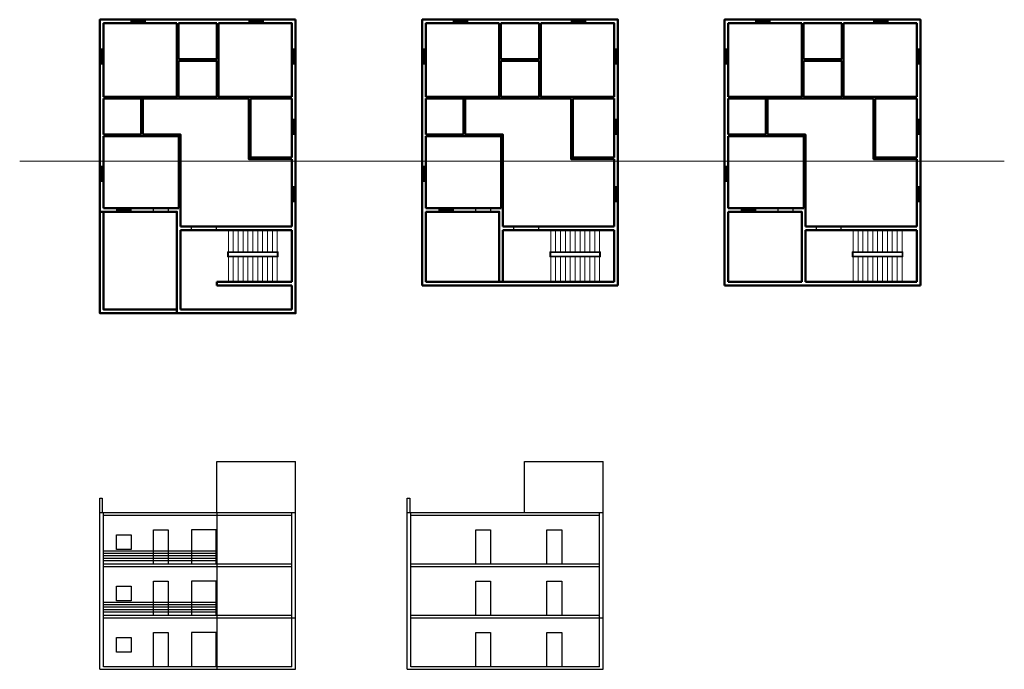
# Model space of a CAD drawing. Units: feet. Extents: x -965 to 1449, y -3391 to -1798.
import ezdxf

# ---------------------------------------------------------------- set-up
doc = ezdxf.new("R2010")
doc.units = ezdxf.units.FT
for name, color, linetype, lineweight in [('A-DOOR', 3, 'Continuous', 25), ('A-ELEV', 7, 'Continuous', 25), ('A-FLOR-STRS', 6, 'Continuous', 18), ('A-GLAZ', 4, 'Continuous', 25), ('A-GRID', 8, 'Continuous', 13), ('A-WALL', 7, 'Continuous', 50)]:
    doc.layers.add(name, color=color, linetype=linetype, lineweight=lineweight)

# ---------------------------------------------------------------- blocks, each defined once
blk = doc.blocks.new('WIN-1200')
for p, q in [((-765.9, -1906), (-765.9, -1870)), ((-764.2, -1906), (-764.2, -1870)), ((-762.5, -1906), (-762.5, -1870))]:
    blk.add_line(p, q)
blk.add_lwpolyline([(-768.7, -1906), (-759.7, -1906), (-759.7, -1870), (-768.7, -1870)], close=True)
blk = doc.blocks.new('ELEV-DOOR')
for p, q in [((0, 0), (0, 84)), ((0, 84), (36, 84)), ((36, 84), (36, 0))]:
    blk.add_line(p, q)
blk = doc.blocks.new('ELEV-WIN-SQ')
for p, q in [((0, 0), (0, 36)), ((0, 36), (36, 36)), ((36, 36), (36, 0)), ((36, 0), (0, 0))]:
    blk.add_line(p, q)
blk = doc.blocks.new('ELEV-DOOR-WIDE')
for p, q in [((60, 84), (0, 84)), ((0, 84), (0, 0)), ((60, 0), (60, 84))]:
    blk.add_line(p, q)

msp = doc.modelspace()

# ---------------------------------------------------------------- linework, layer by layer
at = {"layer": 'A-DOOR'}
for points in [[(-477.7, -1836.7), (-481.7, -1836.7), (-481.7, -1812.7), (-477.7, -1812.7)], [(312.6, -1836.7), (308.6, -1836.7), (308.6, -1812.7), (312.6, -1812.7)], [(1054.2, -1836.7), (1050.2, -1836.7), (1050.2, -1812.7), (1054.2, -1812.7)], [(-575.7, -1980.6), (-579.7, -1980.6), (-579.7, -1956.6), (-575.7, -1956.6)], [(214.6, -1980.6), (210.6, -1980.6), (210.6, -1956.6), (214.6, -1956.6)], [(956.2, -1980.6), (952.2, -1980.6), (952.2, -1956.6), (956.2, -1956.6)], [(-605, -1986.7), (-605, -1990.7), (-641, -1990.7), (-641, -1986.7)], [(-426.7, -1986.7), (-426.7, -1990.7), (-462.7, -1990.7), (-462.7, -1986.7)], [(185.3, -1986.7), (185.3, -1990.7), (149.3, -1990.7), (149.3, -1986.7)], [(363.6, -1986.7), (363.6, -1990.7), (327.6, -1990.7), (327.6, -1986.7)], [(926.9, -1986.7), (926.9, -1990.7), (890.9, -1990.7), (890.9, -1986.7)], [(1105.2, -1986.7), (1105.2, -1990.7), (1069.2, -1990.7), (1069.2, -1986.7)], [(-663.7, -2047.5), (-667.7, -2047.5), (-667.7, -2023.5), (-663.7, -2023.5)], [(126.6, -2047.5), (122.6, -2047.5), (122.6, -2023.5), (126.6, -2023.5)], [(868.2, -2047.5), (864.2, -2047.5), (864.2, -2023.5), (868.2, -2023.5)], [(-601.2, -2079.7), (-601.2, -2083.7), (-637.2, -2083.7), (-637.2, -2079.7)], [(-403.6, -2087.8), (-399.6, -2087.8), (-399.6, -2123.8), (-403.6, -2123.8)], [(189.1, -2079.7), (189.1, -2083.7), (153, -2083.7), (153, -2079.7)], [(386.7, -2087.8), (390.7, -2087.8), (390.7, -2123.8), (386.7, -2123.8)], [(930.6, -2079.7), (930.6, -2083.7), (894.6, -2083.7), (894.6, -2079.7)], [(1128.3, -2087.8), (1132.3, -2087.8), (1132.3, -2123.8), (1128.3, -2123.8)], [(-483.8, -2305.4), (-483.8, -2314.4), (-543.8, -2314.4), (-543.8, -2305.4)], [(306.5, -2305.4), (306.5, -2314.4), (246.5, -2314.4), (246.5, -2305.4)], [(1048.1, -2305.4), (1048.1, -2314.4), (988.1, -2314.4), (988.1, -2305.4)]]:
    msp.add_lwpolyline(points, close=True, dxfattribs=at)
for points in [[(-637.2, -2268.7), (-637.2, -2259.7), (-601.2, -2259.7), (-601.2, -2268.7)], [(153, -2268.7), (153, -2259.7), (189.1, -2259.7), (189.1, -2268.7)], [(894.6, -2268.7), (894.6, -2259.7), (930.6, -2259.7), (930.6, -2268.7)]]:
    msp.add_lwpolyline(points, dxfattribs=at)
at = {"layer": 'A-ELEV'}
for p, q in [((-481.5, -3007.2), (-481.5, -2881.2)), ((-481.5, -2881.2), (-288.7, -2881.2)), ((-288.7, -3391.2), (-288.7, -2881.2)), ((272.1, -3007.2), (272.1, -2881.2)), ((272.1, -2881.2), (465, -2881.2)), ((465, -3391.2), (465, -2881.2)), ((-768.7, -3007.2), (-768.7, -2971.2)), ((-768.7, -2971.2), (-762.7, -2971.2)), ((-762.7, -2971.2), (-762.7, -3007.2)), ((-15, -3007.2), (-15, -2971.2)), ((-15, -2971.2), (-9, -2971.2)), ((-9, -2971.2), (-9, -3007.2)), ((-288.7, -3007.2), (-768.7, -3007.2)), ((-768.7, -3391.2), (-768.7, -3007.2)), ((-759.7, -3385.2), (-759.7, -3007.2)), ((-759.7, -3013.2), (-297.7, -3013.2)), ((-481.5, -3007.2), (-481.5, -3391.2)), ((-297.7, -3385.2), (-297.7, -3007.2)), ((465, -3007.2), (-15, -3007.2)), ((-15, -3391.2), (-15, -3007.2)), ((-6, -3385.2), (-6, -3007.2)), ((-6, -3013.2), (456, -3013.2)), ((456, -3385.2), (456, -3007.2)), ((-481.5, -3124.9), (-759.7, -3124.9)), ((-297.7, -3133.2), (-759.7, -3133.2)), ((-297.7, -3133.2), (-759.7, -3133.2)), ((456, -3133.2), (-6, -3133.2)), ((456, -3133.2), (-6, -3133.2)), ((-759.7, -3139.2), (-297.7, -3139.2)), ((-759.7, -3139.2), (-297.7, -3139.2)), ((-6, -3139.2), (456, -3139.2)), ((-6, -3139.2), (456, -3139.2)), ((-481.5, -3250.9), (-759.7, -3250.9)), ((-297.7, -3259.2), (-759.7, -3259.2)), ((-297.7, -3259.2), (-759.7, -3259.2)), ((-759.7, -3265.2), (-288.7, -3265.2)), ((-759.7, -3265.2), (-297.7, -3265.2)), ((456, -3259.2), (-6, -3259.2)), ((456, -3259.2), (-6, -3259.2)), ((-6, -3265.2), (465, -3265.2)), ((-6, -3265.2), (456, -3265.2)), ((-768.7, -3391.2), (-288.7, -3391.2)), ((-297.7, -3385.2), (-759.7, -3385.2)), ((-15, -3391.2), (465, -3391.2)), ((456, -3385.2), (-6, -3385.2))]:
    msp.add_line(p, q, dxfattribs=at)
for points in [[(-481.5, -3107.3), (-759.7, -3107.3), (-759.7, -3100.3), (-481.5, -3100.3)], [(-481.5, -3119.1), (-759.7, -3119.1), (-759.7, -3112.2), (-481.5, -3112.2)], [(-481.5, -3233.3), (-759.7, -3233.3), (-759.7, -3226.3), (-481.5, -3226.3)], [(-481.5, -3245.1), (-759.7, -3245.1), (-759.7, -3238.2), (-481.5, -3238.2)]]:
    msp.add_lwpolyline(points, close=True, dxfattribs=at)
at = {"layer": 'A-FLOR-STRS'}
for p, q in [((-453.7, -2314.4), (-453.7, -2367.2)), ((-441.7, -2314.4), (-441.7, -2367.2)), ((-429.7, -2314.4), (-429.7, -2367.2)), ((-417.7, -2314.4), (-417.7, -2367.2)), ((-405.7, -2314.4), (-405.7, -2367.2)), ((-393.7, -2314.4), (-393.7, -2367.2)), ((-381.7, -2314.4), (-381.7, -2367.2)), ((-369.7, -2314.4), (-369.7, -2367.2)), ((-357.7, -2314.4), (-357.7, -2367.2)), ((-345.7, -2314.4), (-345.7, -2367.2)), ((-333.7, -2314.4), (-333.7, -2367.2)), ((336.6, -2314.4), (336.6, -2367.2)), ((348.6, -2314.4), (348.6, -2367.2)), ((360.6, -2314.4), (360.6, -2367.2)), ((372.6, -2314.4), (372.6, -2367.2)), ((384.6, -2314.4), (384.6, -2367.2)), ((396.6, -2314.4), (396.6, -2367.2)), ((408.6, -2314.4), (408.6, -2367.2)), ((420.6, -2314.4), (420.6, -2367.2)), ((432.6, -2314.4), (432.6, -2367.2)), ((444.6, -2314.4), (444.6, -2367.2)), ((456.6, -2314.4), (456.6, -2367.2)), ((1078.2, -2314.4), (1078.2, -2367.2)), ((1090.2, -2314.4), (1090.2, -2367.2)), ((1102.2, -2314.4), (1102.2, -2367.2)), ((1114.2, -2314.4), (1114.2, -2367.2)), ((1126.2, -2314.4), (1126.2, -2367.2)), ((1138.2, -2314.4), (1138.2, -2367.2)), ((1150.2, -2314.4), (1150.2, -2367.2)), ((1162.2, -2314.4), (1162.2, -2367.2)), ((1174.2, -2314.4), (1174.2, -2367.2)), ((1186.2, -2314.4), (1186.2, -2367.2)), ((1198.2, -2314.4), (1198.2, -2367.2)), ((-453.7, -2369.2), (-453.7, -2377.7)), ((-453.7, -2379.7), (-453.7, -2440.9)), ((-441.7, -2379.7), (-441.7, -2440.9)), ((-429.7, -2379.7), (-429.7, -2440.9)), ((-417.7, -2379.7), (-417.7, -2440.9)), ((-405.7, -2379.7), (-405.7, -2440.9)), ((-393.7, -2379.7), (-393.7, -2440.9)), ((-381.7, -2379.7), (-381.7, -2440.9)), ((-369.7, -2379.7), (-369.7, -2440.9)), ((-357.7, -2379.7), (-357.7, -2440.9)), ((-345.7, -2379.7), (-345.7, -2440.9)), ((-333.7, -2369.2), (-333.7, -2377.7)), ((-333.7, -2379.7), (-333.7, -2440.9)), ((336.6, -2369.2), (336.6, -2377.7)), ((336.6, -2379.7), (336.6, -2440.9)), ((348.6, -2379.7), (348.6, -2440.9)), ((360.6, -2379.7), (360.6, -2440.9)), ((372.6, -2379.7), (372.6, -2440.9)), ((384.6, -2379.7), (384.6, -2440.9)), ((396.6, -2379.7), (396.6, -2440.9)), ((408.6, -2379.7), (408.6, -2440.9)), ((420.6, -2379.7), (420.6, -2440.9)), ((432.6, -2379.7), (432.6, -2440.9)), ((444.6, -2379.7), (444.6, -2440.9)), ((456.6, -2369.2), (456.6, -2377.7)), ((456.6, -2379.7), (456.6, -2440.9)), ((1078.2, -2369.2), (1078.2, -2377.7)), ((1078.2, -2379.7), (1078.2, -2440.9)), ((1090.2, -2379.7), (1090.2, -2440.9)), ((1102.2, -2379.7), (1102.2, -2440.9)), ((1114.2, -2379.7), (1114.2, -2440.9)), ((1126.2, -2379.7), (1126.2, -2440.9)), ((1138.2, -2379.7), (1138.2, -2440.9)), ((1150.2, -2379.7), (1150.2, -2440.9)), ((1162.2, -2379.7), (1162.2, -2440.9)), ((1174.2, -2379.7), (1174.2, -2440.9)), ((1186.2, -2379.7), (1186.2, -2440.9)), ((1198.2, -2369.2), (1198.2, -2377.7)), ((1198.2, -2379.7), (1198.2, -2440.9))]:
    msp.add_line(p, q, dxfattribs=at)
for points in [[(-331.7, -2379.7), (-455.7, -2379.7), (-455.7, -2367.2), (-331.7, -2367.2)], [(458.6, -2379.7), (334.6, -2379.7), (334.6, -2367.2), (458.6, -2367.2)], [(1200.2, -2379.7), (1076.2, -2379.7), (1076.2, -2367.2), (1200.2, -2367.2)]]:
    msp.add_lwpolyline(points, close=True, dxfattribs=at)
for points in [[(-453.7, -2369.2), (-333.7, -2369.2)], [(-333.7, -2377.7), (-453.7, -2377.7)], [(336.6, -2369.2), (456.6, -2369.2)], [(456.6, -2377.7), (336.6, -2377.7)], [(1078.2, -2369.2), (1198.2, -2369.2)], [(1198.2, -2377.7), (1078.2, -2377.7)]]:
    msp.add_lwpolyline(points, dxfattribs=at)
at = {"layer": 'A-GRID'}
msp.add_line((-965.3, -2144.4), (1448.8, -2144.4), dxfattribs=at)
at = {"layer": 'A-WALL'}
for p, q in [((-481.7, -1894.7), (-575.7, -1894.7)), ((-575.7, -1898.7), (-481.7, -1898.7)), ((308.6, -1894.7), (214.6, -1894.7)), ((214.6, -1898.7), (308.6, -1898.7)), ((1050.2, -1894.7), (956.2, -1894.7)), ((956.2, -1898.7), (1050.2, -1898.7)), ((-667.7, -1990.7), (-667.7, -2079.7)), ((-663.7, -1990.7), (-663.7, -2079.7)), ((-481.7, -1986.7), (-575.7, -1986.7)), ((-575.7, -1990.7), (-481.7, -1990.7)), ((122.6, -1990.7), (122.6, -2079.7)), ((126.6, -1990.7), (126.6, -2079.7)), ((308.6, -1986.7), (214.6, -1986.7)), ((214.6, -1990.7), (308.6, -1990.7)), ((864.2, -1990.7), (864.2, -2079.7)), ((868.2, -1990.7), (868.2, -2079.7)), ((1050.2, -1986.7), (956.2, -1986.7)), ((956.2, -1990.7), (1050.2, -1990.7)), ((-297.7, -2305.4), (-570.7, -2305.4)), ((-297.7, -2314.4), (-570.7, -2314.4)), ((-297.7, -2314.4), (-297.7, -2440.9)), ((492.6, -2305.4), (219.6, -2305.4)), ((492.6, -2314.4), (219.6, -2314.4)), ((492.6, -2314.4), (492.6, -2440.9)), ((1234.2, -2305.4), (961.2, -2305.4)), ((1234.2, -2314.4), (961.2, -2314.4)), ((1234.2, -2314.4), (1234.2, -2440.9)), ((-297.7, -2440.9), (-481.5, -2440.9)), ((-481.5, -2440.9), (-481.5, -2449.9)), ((-481.5, -2449.9), (-297.7, -2449.9)), ((308.7, -2449.9), (21.6, -2449.9)), ((492.6, -2440.9), (30.6, -2440.9)), ((308.7, -2449.9), (501.6, -2449.9)), ((763.2, -2449.9), (1243.2, -2449.9)), ((952.2, -2440.9), (772.2, -2440.9)), ((1234.2, -2440.9), (961.2, -2440.9)), ((-570.7, -2508.7), (-297.7, -2508.7))]:
    msp.add_line(p, q, dxfattribs=at)
msp.add_lwpolyline([(-288.7, -1797.7), (-288.7, -2517.7), (-768.7, -2517.7), (-768.7, -1797.7)], close=True, dxfattribs=at)
for points in [[(-579.7, -1806.7), (-579.7, -1986.7), (-759.7, -1986.7)], [(-759.7, -1986.7), (-759.7, -1806.7), (-579.7, -1806.7)], [(-575.7, -1806.7), (-481.7, -1806.7)], [(-575.7, -1806.7), (-575.7, -1894.7)], [(-481.7, -1806.7), (-481.7, -1894.7)], [(-477.7, -1806.7), (-477.7, -1986.7), (-297.7, -1986.7)], [(-477.7, -1806.7), (-297.7, -1806.7), (-297.7, -1986.7)], [(21.6, -2449.9), (21.6, -1797.7), (501.6, -1797.7), (501.6, -2449.9)], [(30.6, -1986.7), (30.6, -1806.7), (210.6, -1806.7)], [(210.6, -1806.7), (210.6, -1986.7), (30.6, -1986.7)], [(214.6, -1806.7), (308.6, -1806.7)], [(214.6, -1806.7), (214.6, -1894.7)], [(308.6, -1806.7), (308.6, -1894.7)], [(312.6, -1806.7), (492.6, -1806.7), (492.6, -1986.7)], [(312.6, -1806.7), (312.6, -1986.7), (492.6, -1986.7)], [(763.2, -2449.9), (763.2, -1797.7), (1243.2, -1797.7), (1243.2, -2449.9)], [(772.2, -1986.7), (772.2, -1806.7), (952.2, -1806.7)], [(952.2, -1806.7), (952.2, -1986.7), (772.2, -1986.7)], [(956.2, -1806.7), (1050.2, -1806.7)], [(956.2, -1806.7), (956.2, -1894.7)], [(1050.2, -1806.7), (1050.2, -1894.7)], [(1054.2, -1806.7), (1234.2, -1806.7), (1234.2, -1986.7)], [(1054.2, -1806.7), (1054.2, -1986.7), (1234.2, -1986.7)], [(-575.7, -1898.7), (-575.7, -1986.7)], [(-481.7, -1898.7), (-481.7, -1986.7)], [(214.6, -1898.7), (214.6, -1986.7)], [(308.6, -1898.7), (308.6, -1986.7)], [(956.2, -1898.7), (956.2, -1986.7)], [(1050.2, -1898.7), (1050.2, -1986.7)], [(-575.7, -1990.7), (-759.7, -1990.7)], [(-759.7, -2079.7), (-759.7, -1990.7)], [(-481.7, -1990.7), (-403.6, -1990.7)], [(-403.6, -1990.7), (-403.6, -2139.7), (-297.7, -2139.7)], [(-399.6, -1990.7), (-399.6, -2135.7), (-297.7, -2135.7)], [(-399.6, -1990.7), (-297.7, -1990.7)], [(-297.7, -1990.7), (-297.7, -2135.7)], [(30.6, -2079.7), (30.6, -1990.7)], [(214.6, -1990.7), (30.6, -1990.7)], [(308.6, -1990.7), (386.7, -1990.7)], [(386.7, -1990.7), (386.7, -2139.7), (492.6, -2139.7)], [(390.7, -1990.7), (492.6, -1990.7)], [(390.7, -1990.7), (390.7, -2135.7), (492.6, -2135.7)], [(492.6, -1990.7), (492.6, -2135.7)], [(772.2, -2079.7), (772.2, -1990.7)], [(956.2, -1990.7), (772.2, -1990.7)], [(1050.2, -1990.7), (1128.3, -1990.7)], [(1128.3, -1990.7), (1128.3, -2139.7), (1234.2, -2139.7)], [(1132.3, -1990.7), (1234.2, -1990.7)], [(1132.3, -1990.7), (1132.3, -2135.7), (1234.2, -2135.7)], [(1234.2, -1990.7), (1234.2, -2135.7)], [(-667.7, -2079.7), (-759.7, -2079.7)], [(-759.7, -2259.7), (-759.7, -2083.7)], [(-574.7, -2259.7), (-574.7, -2083.7), (-759.7, -2083.7)], [(-570.7, -2259.7), (-570.7, -2079.7), (-663.7, -2079.7)], [(122.6, -2079.7), (30.6, -2079.7)], [(30.6, -2259.7), (30.6, -2083.7)], [(215.6, -2259.7), (215.6, -2083.7), (30.6, -2083.7)], [(219.6, -2259.7), (219.6, -2079.7), (126.6, -2079.7)], [(864.2, -2079.7), (772.2, -2079.7)], [(772.2, -2259.7), (772.2, -2083.7)], [(957.2, -2259.7), (957.2, -2083.7), (772.2, -2083.7)], [(961.2, -2259.7), (961.2, -2079.7), (868.2, -2079.7)], [(-297.7, -2139.7), (-297.7, -2305.4)], [(492.6, -2139.7), (492.6, -2305.4)], [(1234.2, -2139.7), (1234.2, -2305.4)], [(-768.7, -2268.7), (-579.7, -2268.7), (-579.7, -2517.7)], [(-759.7, -2259.7), (-574.7, -2259.7)], [(-579.7, -2508.7), (-759.7, -2508.7), (-759.7, -2268.7)], [(-570.7, -2259.7), (-570.7, -2305.4)], [(30.6, -2259.7), (215.6, -2259.7)], [(30.6, -2268.7), (210.6, -2268.7), (210.6, -2440.9)], [(30.6, -2440.9), (30.6, -2268.7)], [(219.6, -2259.7), (219.6, -2305.4)], [(772.2, -2259.7), (957.2, -2259.7)], [(772.2, -2268.7), (952.2, -2268.7), (952.2, -2440.9)], [(772.2, -2440.9), (772.2, -2268.7)], [(961.2, -2259.7), (961.2, -2305.4)], [(-570.7, -2314.4), (-570.7, -2508.7)], [(-297.7, -2314.4), (-297.7, -2440.9)], [(219.6, -2314.4), (219.6, -2440.9)], [(492.6, -2314.4), (492.6, -2440.9)], [(961.2, -2314.4), (961.2, -2440.9)], [(1234.2, -2314.4), (1234.2, -2440.9)], [(-297.7, -2449.9), (-297.7, -2508.7)]]:
    msp.add_lwpolyline(points, dxfattribs=at)

# ---------------------------------------------------------------- block references
at = {"layer": 'A-ELEV'}
for name, p in [('ELEV-WIN-SQ', (-727.9, -3097.2)), ('ELEV-DOOR', (-637.2, -3133.2)), ('ELEV-DOOR-WIDE', (-543.8, -3133.2)), ('ELEV-DOOR', (153, -3133.2)), ('ELEV-DOOR', (327.6, -3133.2)), ('ELEV-DOOR', (-637.2, -3259.2)), ('ELEV-DOOR-WIDE', (-543.8, -3259.2)), ('ELEV-DOOR', (153, -3259.2)), ('ELEV-DOOR', (327.6, -3259.2)), ('ELEV-WIN-SQ', (-727.9, -3223.2)), ('ELEV-DOOR', (-637.2, -3385.2)), ('ELEV-DOOR-WIDE', (-543.8, -3385.2)), ('ELEV-DOOR', (153, -3385.2)), ('ELEV-DOOR', (327.6, -3385.2)), ('ELEV-WIN-SQ', (-727.9, -3349.2))]:
    msp.add_blockref(name, p, dxfattribs=at)
at = {"layer": 'A-GLAZ'}
for p, rotation in [((-2563, -1038.1), 90.00000000000087), ((-2273.7, -1038.1), 90.00000000000087), ((-1772.7, -1038.1), 90.00000000000087), ((-1483.4, -1038.1), 90.00000000000087), ((-1031.1, -1038.1), 90.0000000000009), ((-741.9, -1038.1), 90.0000000000009), ((-2597.9, -1500.1), 90.00000000000087), ((-1807.6, -1500.1), 90.00000000000088), ((-1066, -1500.1), 90.00000000000087)]:
    msp.add_blockref('WIN-1200', p, dxfattribs=dict(at, rotation=rotation))
for p in [(0, 0), (471, 0), (790.3, 0), (1261.3, 0), (1531.9, 0), (2002.9, 0), (471, -172.7), (1261.3, -172.7), (2002.9, -172.7), (0, -287.8), (790.3, -287.8), (1531.9, -287.8), (471, -338.1), (1261.3, -338.1), (2002.9, -338.1)]:
    msp.add_blockref('WIN-1200', p, dxfattribs=at)

doc.saveas('drawing.dxf')
